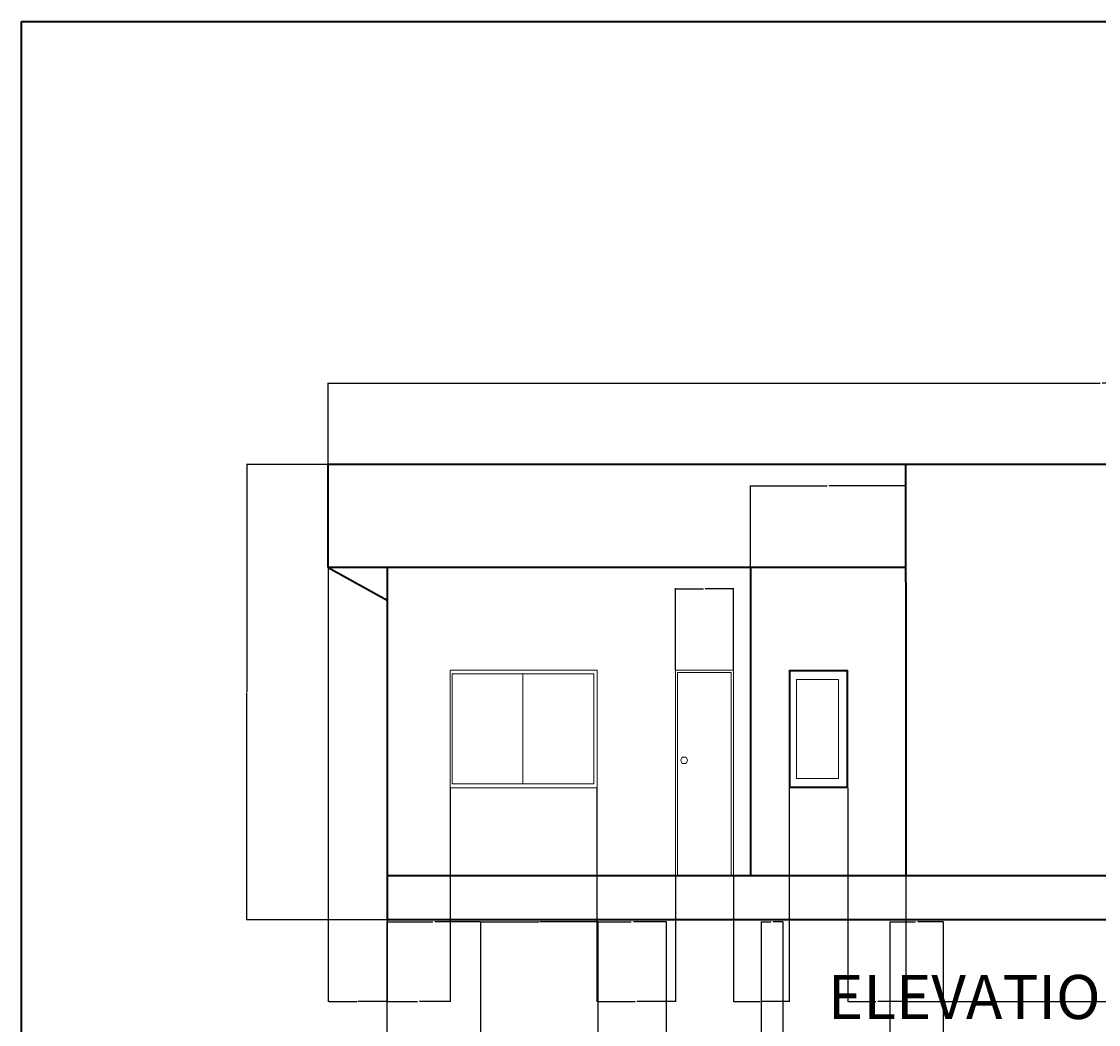
# Model space of a CAD drawing. Units: inches. Extents: x 392 to 1254, y 1207 to 2665.
# Tile 11 of 15: x 392 to 832, y 2255 to 2665. Entities that reach past the tile are written whole.
import ezdxf

# ---------------------------------------------------------------- set-up
doc = ezdxf.new("R2010")
doc.units = ezdxf.units.IN
for name, color, linetype, lineweight in [('A-ANNO-DIMS', 2, 'Continuous', 18), ('A-ANNO-TEXT', 7, 'Continuous', 25), ('A-ANNO-TTLB', 7, 'Continuous', 35), ('A-ELEV', 7, 'Continuous', 35), ('A-ELEV-OPEN', 4, 'Continuous', 18)]:
    doc.layers.add(name, color=color, linetype=linetype, lineweight=lineweight)
doc.styles.get("Standard").update_dxf_attribs({"font": 'arial.ttf'})
doc.dimstyles.get("Standard").update_dxf_attribs({"dimtxt": 0.18, "dimasz": 0.18, "dimexe": 0.18, "dimexo": 0.0625, "dimgap": 0.09, "dimtad": 0, "dimtih": 1, "dimtoh": 1, "dimdec": 4, "dimzin": 0, "dimdsep": 46, "dimtxsty": 'Standard', "dimcen": 0.09, "dimadec": 0, "dimazin": 0, "dimtfac": 1, "dimtdec": 4, "dimtofl": 0, "dimtmove": 0, "dimatfit": 3, "dimfxl": 1, "dimtolj": 1, "dimtzin": 0, "dimarcsym": 0})

# ---------------------------------------------------------------- blocks, each defined once
blk = doc.blocks.new('*D44')
at = {"layer": 'A-ANNO-DIMS', "color": 0, "lineweight": -2, "transparency": 16777216}
for p, q in [((541.28, 2229.36), (541.28, 2297.33)), ((541.46, 2297.15), (560.01, 2297.15)), ((579.35, 2297.15), (560.8, 2297.15)), ((579.53, 2229.36), (579.53, 2297.33))]:
    blk.add_line(p, q, dxfattribs=at)
at = {"layer": 'A-ANNO-DIMS', "color": 0, "transparency": 16777216}
for points in [[(541.46, 2297.18), (541.46, 2297.12), (541.28, 2297.15)], [(579.35, 2297.18), (579.35, 2297.12), (579.53, 2297.15)]]:
    blk.add_solid(points, dxfattribs=at)
at = {"layer": 'Defpoints', "color": 0, "transparency": 16777216}
for p in [(579.53, 2297.15), (541.28, 2229.3), (579.53, 2229.3)]:
    blk.add_point(p, dxfattribs=at)
at = {"layer": 'A-ANNO-DIMS', "color": 0, "transparency": 16777216, "insert": (560.41, 2297.15), "char_height": 0.18, "attachment_point": 5}
blk.add_mtext('\\A1;38.25', dxfattribs=at)
blk = doc.blocks.new('*D45')
at = {"layer": 'A-ANNO-DIMS', "color": 0, "lineweight": -2, "transparency": 16777216}
for p, q in [((579.53, 2229.36), (579.53, 2297.33)), ((579.71, 2297.15), (603.31, 2297.15)), ((627.35, 2297.15), (603.75, 2297.15)), ((627.53, 2229.36), (627.53, 2297.33))]:
    blk.add_line(p, q, dxfattribs=at)
at = {"layer": 'A-ANNO-DIMS', "color": 0, "transparency": 16777216}
for points in [[(579.71, 2297.18), (579.71, 2297.12), (579.53, 2297.15)], [(627.35, 2297.18), (627.35, 2297.12), (627.53, 2297.15)]]:
    blk.add_solid(points, dxfattribs=at)
at = {"layer": 'Defpoints', "color": 0, "transparency": 16777216}
for p in [(627.53, 2297.15), (579.53, 2229.3), (627.53, 2229.3)]:
    blk.add_point(p, dxfattribs=at)
at = {"layer": 'A-ANNO-DIMS', "color": 0, "transparency": 16777216, "insert": (603.53, 2297.15), "char_height": 0.18, "attachment_point": 5}
blk.add_mtext('\\A1;48', dxfattribs=at)
blk = doc.blocks.new('*D46')
at = {"layer": 'A-ANNO-DIMS', "color": 0, "lineweight": -2, "transparency": 16777216}
for p, q in [((627.53, 2229.36), (627.53, 2297.33)), ((627.71, 2297.15), (641.02, 2297.15)), ((655.26, 2297.15), (641.95, 2297.15)), ((655.44, 2229.36), (655.44, 2297.33))]:
    blk.add_line(p, q, dxfattribs=at)
at = {"layer": 'A-ANNO-DIMS', "color": 0, "transparency": 16777216}
for points in [[(627.71, 2297.18), (627.71, 2297.12), (627.53, 2297.15)], [(655.26, 2297.18), (655.26, 2297.12), (655.44, 2297.15)]]:
    blk.add_solid(points, dxfattribs=at)
at = {"layer": 'Defpoints', "color": 0, "transparency": 16777216}
for p in [(655.44, 2297.15), (627.53, 2229.3), (655.44, 2229.3)]:
    blk.add_point(p, dxfattribs=at)
at = {"layer": 'A-ANNO-DIMS', "color": 0, "transparency": 16777216, "insert": (641.49, 2297.15), "char_height": 0.18, "attachment_point": 5}
blk.add_mtext('\\A1;27.913', dxfattribs=at)
blk = doc.blocks.new('*D54')
at = {"layer": 'A-ANNO-DIMS', "color": 0, "lineweight": -2, "transparency": 16777216}
for p, q in [((517.28, 2483.97), (517.28, 2517.38)), ((517.46, 2517.2), (832.64, 2517.2)), ((1148.6, 2517.2), (833.43, 2517.2)), ((1148.78, 2483.97), (1148.78, 2517.38))]:
    blk.add_line(p, q, dxfattribs=at)
at = {"layer": 'A-ANNO-DIMS', "color": 0, "transparency": 16777216}
for points in [[(517.46, 2517.23), (517.46, 2517.17), (517.28, 2517.2)], [(1148.6, 2517.23), (1148.6, 2517.17), (1148.78, 2517.2)]]:
    blk.add_solid(points, dxfattribs=at)
at = {"layer": 'Defpoints', "color": 0, "transparency": 16777216}
for p in [(1148.78, 2517.2), (517.28, 2483.9), (1148.78, 2483.9)]:
    blk.add_point(p, dxfattribs=at)
at = {"layer": 'A-ANNO-DIMS', "color": 0, "transparency": 16777216, "insert": (833.03, 2517.2), "char_height": 0.18, "attachment_point": 5}
blk.add_mtext('\\A1;631.5', dxfattribs=at)
blk = doc.blocks.new('*D55')
at = {"layer": 'A-ANNO-DIMS', "color": 0, "lineweight": -2, "transparency": 16777216}
for p, q in [((517.22, 2483.9), (483.8, 2483.9)), ((483.98, 2483.72), (483.98, 2391.08)), ((483.98, 2298.08), (483.98, 2390.72)), ((541.22, 2297.9), (483.8, 2297.9))]:
    blk.add_line(p, q, dxfattribs=at)
at = {"layer": 'A-ANNO-DIMS', "color": 0, "transparency": 16777216}
for points in [[(483.95, 2483.72), (484.01, 2483.72), (483.98, 2483.9)], [(483.95, 2298.08), (484.01, 2298.08), (483.98, 2297.9)]]:
    blk.add_solid(points, dxfattribs=at)
at = {"layer": 'Defpoints', "color": 0, "transparency": 16777216}
for p in [(483.98, 2483.9), (517.28, 2483.9), (541.28, 2297.9)]:
    blk.add_point(p, dxfattribs=at)
at = {"layer": 'A-ANNO-DIMS', "color": 0, "transparency": 16777216, "insert": (483.98, 2390.9), "char_height": 0.18, "attachment_point": 5}
blk.add_mtext('\\A1;186', dxfattribs=at)
blk = doc.blocks.new('*D60')
at = {"layer": 'A-ANNO-DIMS', "color": 0, "lineweight": -2, "transparency": 16777216}
for p, q in [((517.28, 2441.84), (517.28, 2264.42)), ((541.28, 2297.84), (541.28, 2264.42)), ((517.46, 2264.6), (529.06, 2264.6)), ((541.1, 2264.6), (529.5, 2264.6))]:
    blk.add_line(p, q, dxfattribs=at)
at = {"layer": 'A-ANNO-DIMS', "color": 0, "transparency": 16777216}
for points in [[(517.46, 2264.63), (517.46, 2264.57), (517.28, 2264.6)], [(541.1, 2264.63), (541.1, 2264.57), (541.28, 2264.6)]]:
    blk.add_solid(points, dxfattribs=at)
at = {"layer": 'Defpoints', "color": 0, "transparency": 16777216}
for p in [(517.28, 2441.9), (541.28, 2297.9), (541.28, 2264.6)]:
    blk.add_point(p, dxfattribs=at)
at = {"layer": 'A-ANNO-DIMS', "color": 0, "transparency": 16777216, "insert": (529.28, 2264.6), "char_height": 0.18, "attachment_point": 5}
blk.add_mtext('\\A1;24', dxfattribs=at)
blk = doc.blocks.new('*D61')
at = {"layer": 'A-ANNO-DIMS', "color": 0, "lineweight": -2, "transparency": 16777216}
for p, q in [((689.78, 2441.97), (689.78, 2475.38)), ((689.96, 2475.2), (721.16, 2475.2)), ((753.11, 2475.2), (721.91, 2475.2)), ((753.29, 2441.97), (753.29, 2475.38))]:
    blk.add_line(p, q, dxfattribs=at)
at = {"layer": 'A-ANNO-DIMS', "color": 0, "transparency": 16777216}
for points in [[(689.96, 2475.23), (689.96, 2475.17), (689.78, 2475.2)], [(753.11, 2475.23), (753.11, 2475.17), (753.29, 2475.2)]]:
    blk.add_solid(points, dxfattribs=at)
at = {"layer": 'Defpoints', "color": 0, "transparency": 16777216}
for p in [(753.29, 2475.2), (689.78, 2441.9), (753.29, 2441.9)]:
    blk.add_point(p, dxfattribs=at)
at = {"layer": 'A-ANNO-DIMS', "color": 0, "transparency": 16777216, "insert": (721.53, 2475.2), "char_height": 0.18, "attachment_point": 5}
blk.add_mtext('\\A1;63.51', dxfattribs=at)
blk = doc.blocks.new('*D63')
at = {"layer": 'A-ANNO-DIMS', "color": 0, "lineweight": -2, "transparency": 16777216}
for p, q in [((567.06, 2351.84), (567.06, 2264.42)), ((541.28, 2297.84), (541.28, 2264.42)), ((541.46, 2264.6), (553.78, 2264.6)), ((566.88, 2264.6), (554.57, 2264.6))]:
    blk.add_line(p, q, dxfattribs=at)
at = {"layer": 'A-ANNO-DIMS', "color": 0, "transparency": 16777216}
for points in [[(541.46, 2264.63), (541.46, 2264.57), (541.28, 2264.6)], [(566.88, 2264.63), (566.88, 2264.57), (567.06, 2264.6)]]:
    blk.add_solid(points, dxfattribs=at)
at = {"layer": 'Defpoints', "color": 0, "transparency": 16777216}
for p in [(567.06, 2351.9), (541.28, 2297.9), (567.06, 2264.6)]:
    blk.add_point(p, dxfattribs=at)
at = {"layer": 'A-ANNO-DIMS', "color": 0, "transparency": 16777216, "insert": (554.17, 2264.6), "char_height": 0.18, "attachment_point": 5}
blk.add_mtext('\\A1;25.78', dxfattribs=at)
blk = doc.blocks.new('*D64')
at = {"layer": 'A-ANNO-DIMS', "color": 0, "lineweight": -2, "transparency": 16777216}
for p, q in [((627.06, 2351.84), (627.06, 2264.42)), ((659.07, 2315.84), (659.07, 2264.42)), ((627.24, 2264.6), (642.6, 2264.6)), ((658.89, 2264.6), (643.53, 2264.6))]:
    blk.add_line(p, q, dxfattribs=at)
at = {"layer": 'A-ANNO-DIMS', "color": 0, "transparency": 16777216}
for points in [[(627.24, 2264.63), (627.24, 2264.57), (627.06, 2264.6)], [(658.89, 2264.63), (658.89, 2264.57), (659.07, 2264.6)]]:
    blk.add_solid(points, dxfattribs=at)
at = {"layer": 'Defpoints', "color": 0, "transparency": 16777216}
for p in [(627.06, 2351.9), (659.07, 2315.9), (659.07, 2264.6)]:
    blk.add_point(p, dxfattribs=at)
at = {"layer": 'A-ANNO-DIMS', "color": 0, "transparency": 16777216, "insert": (643.07, 2264.6), "char_height": 0.18, "attachment_point": 5}
blk.add_mtext('\\A1;32.005', dxfattribs=at)
blk = doc.blocks.new('*D65')
at = {"layer": 'A-ANNO-DIMS', "color": 0, "lineweight": -2, "transparency": 16777216}
for p, q in [((659.07, 2399.97), (659.07, 2433.38)), ((682.77, 2399.97), (682.77, 2433.38)), ((659.25, 2433.2), (670.59, 2433.2)), ((682.59, 2433.2), (671.24, 2433.2))]:
    blk.add_line(p, q, dxfattribs=at)
at = {"layer": 'A-ANNO-DIMS', "color": 0, "transparency": 16777216}
for points in [[(659.25, 2433.23), (659.25, 2433.17), (659.07, 2433.2)], [(682.59, 2433.23), (682.59, 2433.17), (682.77, 2433.2)]]:
    blk.add_solid(points, dxfattribs=at)
at = {"layer": 'Defpoints', "color": 0, "transparency": 16777216}
for p in [(682.77, 2433.2), (659.07, 2399.9), (682.77, 2399.9)]:
    blk.add_point(p, dxfattribs=at)
at = {"layer": 'A-ANNO-DIMS', "color": 0, "transparency": 16777216, "insert": (670.92, 2433.2), "char_height": 0.18, "attachment_point": 5}
blk.add_mtext('\\A1;23.7', dxfattribs=at)
blk = doc.blocks.new('*D66')
at = {"layer": 'A-ANNO-DIMS', "color": 0, "lineweight": -2, "transparency": 16777216}
for p, q in [((705.6, 2351.84), (705.6, 2264.42)), ((682.77, 2315.84), (682.77, 2264.42)), ((682.95, 2264.6), (693.79, 2264.6)), ((705.42, 2264.6), (694.58, 2264.6))]:
    blk.add_line(p, q, dxfattribs=at)
at = {"layer": 'A-ANNO-DIMS', "color": 0, "transparency": 16777216}
for points in [[(682.95, 2264.63), (682.95, 2264.57), (682.77, 2264.6)], [(705.42, 2264.63), (705.42, 2264.57), (705.6, 2264.6)]]:
    blk.add_solid(points, dxfattribs=at)
at = {"layer": 'Defpoints', "color": 0, "transparency": 16777216}
for p in [(705.6, 2351.9), (682.77, 2315.9), (705.6, 2264.6)]:
    blk.add_point(p, dxfattribs=at)
at = {"layer": 'A-ANNO-DIMS', "color": 0, "transparency": 16777216, "insert": (694.18, 2264.6), "char_height": 0.18, "attachment_point": 5}
blk.add_mtext('\\A1;22.83', dxfattribs=at)
blk = doc.blocks.new('*D67')
at = {"layer": 'A-ANNO-DIMS', "color": 0, "lineweight": -2, "transparency": 16777216}
for p, q in [((729.6, 2351.84), (729.6, 2264.42)), ((753.29, 2315.84), (753.29, 2264.42)), ((729.78, 2264.6), (741.05, 2264.6)), ((753.11, 2264.6), (741.84, 2264.6))]:
    blk.add_line(p, q, dxfattribs=at)
at = {"layer": 'A-ANNO-DIMS', "color": 0, "transparency": 16777216}
for points in [[(729.78, 2264.63), (729.78, 2264.57), (729.6, 2264.6)], [(753.11, 2264.63), (753.11, 2264.57), (753.29, 2264.6)]]:
    blk.add_solid(points, dxfattribs=at)
at = {"layer": 'Defpoints', "color": 0, "transparency": 16777216}
for p in [(729.6, 2351.9), (753.29, 2315.9), (753.29, 2264.6)]:
    blk.add_point(p, dxfattribs=at)
at = {"layer": 'A-ANNO-DIMS', "color": 0, "transparency": 16777216, "insert": (741.44, 2264.6), "char_height": 0.18, "attachment_point": 5}
blk.add_mtext('\\A1;23.69', dxfattribs=at)
blk = doc.blocks.new('*D68')
at = {"layer": 'A-ANNO-DIMS', "color": 0, "lineweight": -2, "transparency": 16777216}
for p, q in [((753.29, 2315.84), (753.29, 2264.42)), ((918.49, 2315.84), (918.49, 2264.42)), ((753.47, 2264.6), (835.5, 2264.6)), ((918.31, 2264.6), (836.27, 2264.6))]:
    blk.add_line(p, q, dxfattribs=at)
at = {"layer": 'A-ANNO-DIMS', "color": 0, "transparency": 16777216}
for points in [[(753.47, 2264.63), (753.47, 2264.57), (753.29, 2264.6)], [(918.31, 2264.63), (918.31, 2264.57), (918.49, 2264.6)]]:
    blk.add_solid(points, dxfattribs=at)
at = {"layer": 'Defpoints', "color": 0, "transparency": 16777216}
for p in [(753.29, 2315.9), (918.49, 2315.9), (918.49, 2264.6)]:
    blk.add_point(p, dxfattribs=at)
at = {"layer": 'A-ANNO-DIMS', "color": 0, "transparency": 16777216, "insert": (835.89, 2264.6), "char_height": 0.18, "attachment_point": 5}
blk.add_mtext('\\A1;165.2', dxfattribs=at)
blk = doc.blocks.new('*D76')
at = {"layer": 'A-ANNO-DIMS', "color": 0, "lineweight": -2, "transparency": 16777216}
for p, q in [((694.28, 2224.86), (694.28, 2297.33)), ((694.46, 2297.15), (698.28, 2297.15)), ((702.9, 2297.15), (699.07, 2297.15)), ((703.08, 2224.86), (703.08, 2297.33))]:
    blk.add_line(p, q, dxfattribs=at)
at = {"layer": 'A-ANNO-DIMS', "color": 0, "transparency": 16777216}
for points in [[(694.46, 2297.18), (694.46, 2297.12), (694.28, 2297.15)], [(702.9, 2297.18), (702.9, 2297.12), (703.08, 2297.15)]]:
    blk.add_solid(points, dxfattribs=at)
at = {"layer": 'Defpoints', "color": 0, "transparency": 16777216}
for p in [(703.08, 2297.15), (694.28, 2224.8), (703.08, 2224.8)]:
    blk.add_point(p, dxfattribs=at)
at = {"layer": 'A-ANNO-DIMS', "color": 0, "transparency": 16777216, "insert": (698.68, 2297.15), "char_height": 0.18, "attachment_point": 5}
blk.add_mtext('\\A1;8.795', dxfattribs=at)
blk = doc.blocks.new('*D77')
at = {"layer": 'A-ANNO-DIMS', "color": 0, "lineweight": -2, "transparency": 16777216}
for p, q in [((746.78, 2224.86), (746.78, 2297.33)), ((746.96, 2297.15), (757.21, 2297.15)), ((768.4, 2297.15), (758.14, 2297.15)), ((768.58, 2224.86), (768.58, 2297.33))]:
    blk.add_line(p, q, dxfattribs=at)
at = {"layer": 'A-ANNO-DIMS', "color": 0, "transparency": 16777216}
for points in [[(746.96, 2297.18), (746.96, 2297.12), (746.78, 2297.15)], [(768.4, 2297.18), (768.4, 2297.12), (768.58, 2297.15)]]:
    blk.add_solid(points, dxfattribs=at)
at = {"layer": 'Defpoints', "color": 0, "transparency": 16777216}
for p in [(768.58, 2297.15), (746.78, 2224.8), (768.58, 2224.8)]:
    blk.add_point(p, dxfattribs=at)
at = {"layer": 'A-ANNO-DIMS', "color": 0, "transparency": 16777216, "insert": (757.68, 2297.15), "char_height": 0.18, "attachment_point": 5}
blk.add_mtext('\\A1;21.796', dxfattribs=at)

msp = doc.modelspace()

# ---------------------------------------------------------------- linework, layer by layer
at = {"layer": 'A-ANNO-TTLB'}
msp.add_lwpolyline([(391.939, 2664.8979), (1253.97, 2664.8979), (1253.97, 1207.2611), (391.939, 1207.2611)], close=True, dxfattribs=at)
at = {"layer": 'A-ELEV'}
for p, q in [((1148.7807, 2483.9029), (517.2807, 2483.9029)), ((517.2807, 2441.9029), (517.2807, 2483.9029)), ((753.2885, 2438.9029), (753.2885, 2483.9029)), ((753.2885, 2441.9029), (517.2807, 2441.9029)), ((517.2807, 2441.9029), (541.2807, 2428.4819)), ((541.2807, 2441.9029), (541.2807, 2297.9029)), ((689.7807, 2441.9029), (689.7807, 2315.9029)), ((753.2885, 2435.9029), (753.2885, 2441.9029)), ((753.2885, 2435.9029), (753.2885, 2315.9029)), ((1124.7807, 2315.9029), (541.2807, 2315.9029)), ((1124.7807, 2297.9029), (541.2807, 2297.9029))]:
    msp.add_line(p, q, dxfattribs=at)
at = {"layer": 'A-ELEV-OPEN'}
for p, q in [((567.0628, 2399.9029), (567.0628, 2351.9029)), ((627.0628, 2399.9029), (567.0628, 2399.9029)), ((596.8077, 2398.5002), (596.8077, 2353.5361)), ((627.0628, 2399.9029), (627.0628, 2351.9029)), ((659.068, 2399.9029), (659.068, 2315.9029)), ((682.7672, 2399.9029), (659.068, 2399.9029)), ((682.7672, 2399.9029), (682.7672, 2315.9029)), ((705.598, 2351.9029), (705.598, 2399.9029)), ((705.598, 2399.9029), (729.598, 2399.9029)), ((729.598, 2399.9029), (729.598, 2351.9029)), ((729.598, 2399.9029), (729.598, 2351.9029)), ((627.0628, 2351.9029), (567.0628, 2351.9029)), ((729.598, 2351.9029), (705.598, 2351.9029))]:
    msp.add_line(p, q, dxfattribs=at)
for points in [[(567.904, 2398.5002), (625.7115, 2398.5002), (625.7115, 2353.5361), (567.904, 2353.5361)], [(659.9878, 2398.982), (681.8681, 2398.982), (681.8681, 2315.9029), (659.9878, 2315.9029)], [(705.9348, 2399.5743), (729.1699, 2399.5743), (729.1699, 2352.3115), (705.9348, 2352.3115)], [(708.5132, 2396.0994), (725.7657, 2396.0994), (725.7657, 2355.7407), (708.5132, 2355.7407)]]:
    msp.add_lwpolyline(points, close=True, dxfattribs=at)
msp.add_circle((662.6914, 2363.1179), 1.358, dxfattribs=at)

# ---------------------------------------------------------------- texts
at = {"layer": 'A-ANNO-TEXT', "insert": (721.3964, 2275.4413), "char_height": 18, "attachment_point": 1}
msp.add_mtext_dynamic_manual_height_columns('ELEVATION', width=295.164206, gutter_width=12.5, heights=[0], dxfattribs=at)

# ---------------------------------------------------------------- dimensions: what is measured, and where the dimension line sits
at = {"layer": 'A-ANNO-DIMS'}
for base, p1, p2, override, picture, middle in [((1148.7807, 2517.2029), (517.2807, 2483.9029), (1148.7807, 2483.9029), {"dimdec": 1, "dimlfac": 1, "dimrnd": 0, "dimzin": 0, "dimdsep": 46, "dimlunit": 2}, '*D54', (833.0307, 2517.2029)), ((753.2885, 2475.2029), (689.7807, 2441.9029), (753.2885, 2441.9029), {"dimdec": 2, "dimlfac": 1, "dimrnd": 0, "dimzin": 0, "dimdsep": 46, "dimlunit": 2}, '*D61', (721.5346, 2475.2029)), ((541.2807, 2264.6029), (517.2807, 2441.9029), (541.2807, 2297.9029), {"dimdec": 0, "dimlfac": 1, "dimrnd": 0, "dimzin": 0, "dimdsep": 46, "dimlunit": 2}, '*D60', (529.2807, 2264.6029)), ((682.7672, 2433.2029), (659.068, 2399.9029), (682.7672, 2399.9029), {"dimdec": 1, "dimlfac": 1, "dimrnd": 0, "dimzin": 0, "dimdsep": 46, "dimlunit": 2}, '*D65', (670.9176, 2433.2029)), ((567.0628, 2264.6029), (541.2807, 2297.9029), (567.0628, 2351.9029), {"dimdec": 2, "dimlfac": 1, "dimrnd": 0, "dimzin": 0, "dimdsep": 46, "dimlunit": 2}, '*D63', (554.1717, 2264.6029)), ((659.068, 2264.6029), (627.0628, 2351.9029), (659.068, 2315.9029), {"dimdec": 3, "dimlfac": 1, "dimrnd": 0, "dimzin": 0, "dimdsep": 46, "dimlunit": 2}, '*D64', (643.0654, 2264.6029)), ((705.598, 2264.6029), (682.7672, 2315.9029), (705.598, 2351.9029), {"dimdec": 2, "dimlfac": 1, "dimrnd": 0, "dimzin": 0, "dimdsep": 46, "dimlunit": 2}, '*D66', (694.1826, 2264.6029)), ((753.2885, 2264.6029), (729.598, 2351.9029), (753.2885, 2315.9029), {"dimdec": 2, "dimlfac": 1, "dimrnd": 0, "dimzin": 0, "dimdsep": 46, "dimlunit": 2}, '*D67', (741.4433, 2264.6029)), ((918.4852, 2264.6029), (753.2885, 2315.9029), (918.4852, 2315.9029), {"dimdec": 1, "dimlfac": 1, "dimrnd": 0, "dimzin": 0, "dimdsep": 46, "dimlunit": 2}, '*D68', (835.8869, 2264.6029)), ((579.5309, 2297.1453), (541.2807, 2229.2953), (579.5309, 2229.2953), {"dimdec": 2, "dimlfac": 1, "dimrnd": 0, "dimzin": 0, "dimdsep": 46, "dimlunit": 2}, '*D44', (560.4058, 2297.1453)), ((627.5309, 2297.1453), (579.5309, 2229.2953), (627.5309, 2229.2953), {"dimdec": 0, "dimlfac": 1, "dimrnd": 0, "dimzin": 0, "dimdsep": 46, "dimlunit": 2}, '*D45', (603.5309, 2297.1453)), ((655.4442, 2297.1453), (627.5309, 2229.2953), (655.4442, 2229.2953), {"dimdec": 3, "dimlfac": 1, "dimrnd": 0, "dimzin": 0, "dimdsep": 46, "dimlunit": 2}, '*D46', (641.4875, 2297.1453)), ((703.0758, 2297.1453), (694.2807, 2224.7953), (703.0758, 2224.7953), {"dimdec": 3, "dimlfac": 1, "dimrnd": 0, "dimzin": 0, "dimdsep": 46, "dimlunit": 2}, '*D76', (698.6783, 2297.1453)), ((768.5767, 2297.1453), (746.7807, 2224.7953), (768.5767, 2224.7953), {"dimdec": 3, "dimlfac": 1, "dimrnd": 0, "dimzin": 0, "dimdsep": 46, "dimlunit": 2}, '*D77', (757.6787, 2297.1453))]:
    dim = msp.add_linear_dim(base=base, p1=p1, p2=p2, dimstyle='Standard', override=override, dxfattribs=at)
    dim.commit()
    dim.dimension.update_dxf_attribs({"geometry": picture, "text_midpoint": middle})
dim = msp.add_linear_dim(base=(483.9807, 2483.9029), p1=(541.2807, 2297.9029), p2=(517.2807, 2483.9029), angle=90, dimstyle='Standard', override={"dimdec": 0, "dimlfac": 1, "dimrnd": 0, "dimzin": 0, "dimdsep": 46, "dimlunit": 2}, dxfattribs=at)
dim.commit()
dim.dimension.update_dxf_attribs({"geometry": '*D55', "text_midpoint": (483.9807, 2390.9029)})

doc.saveas('drawing.dxf')
